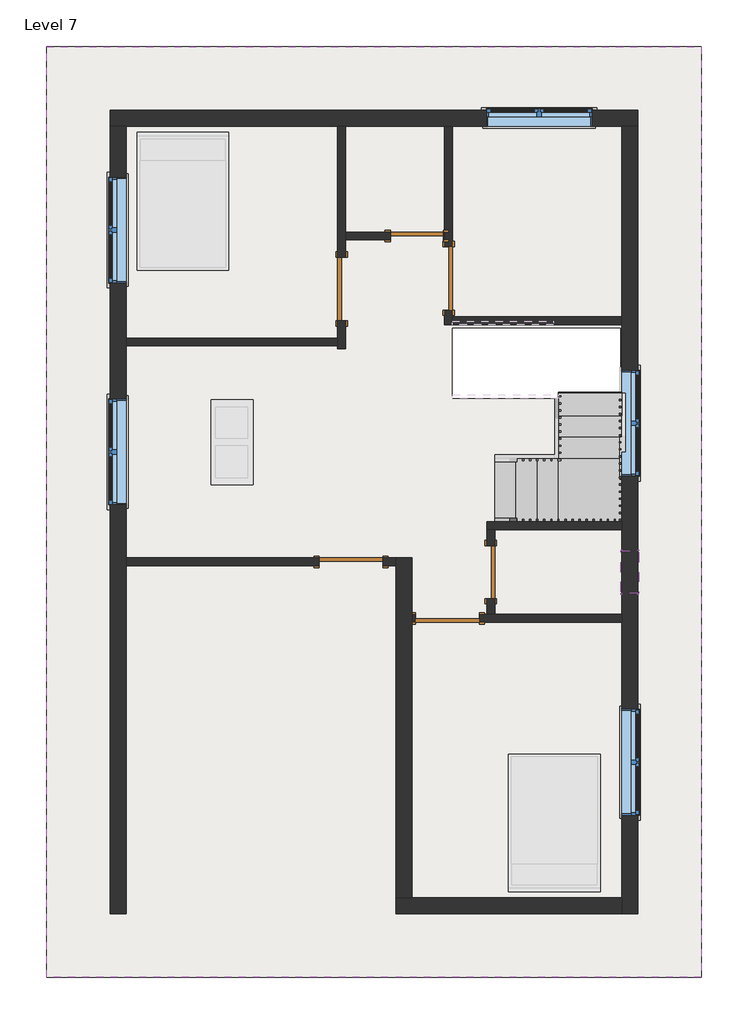
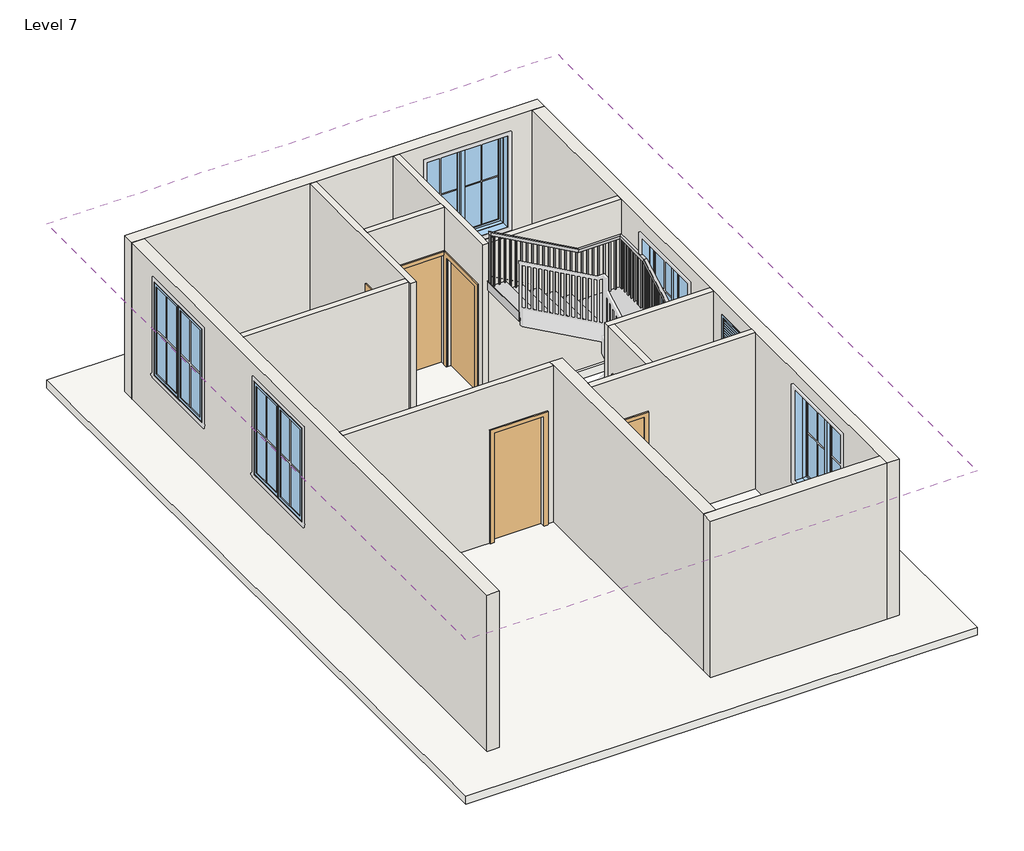
# One storey, part 1 of 2: 14 walls, 6 doors, 6 windows, 2 roofs, 1 railing, 1 slab, 1 stair flight.
# Revit data of these elements (continued)
# Elements 21, 22, 23, 24, 25 (IfcWall, "WALL 9\"")
#   Top Offset = 0' - 0"
#   Base Offset = 0' - 0"
#   Unconnected Height = 10' - 0"
#   wall height = 10' - 0"
#   Phase Created = New Construction
#   Base Constraint = Level 7
#   Materials on its faces: "Default Wall", "Copper"
# Element 26 (IfcWindow, "Window-Casement-Double : WIN 5'")
#   Mark = "31"
#   Window Inset = 0' - 0"
#   Interior Wall Closure = 0' - 2 1/4"
#   Frame Extension = 0' - 0 1/4"
#   Exterior Wall Closure = 0' - 1 1/4"
#   Interior Trim Visibility = yes
#   Exterior Trim Visibility = yes
#   Phase Created = New Construction
#   Materials on its faces: "Wood - Stained", "Glass", "Clad - White"
# Element 27 (IfcWindow, "Window-Casement-Double : WIN 5'")
#   Mark = "32"
#   Window Inset = 0' - 0"
#   Interior Wall Closure = 0' - 2 1/4"
#   Frame Extension = 0' - 0 1/4"
#   Exterior Wall Closure = 0' - 1 1/4"
#   Interior Trim Visibility = yes
#   Exterior Trim Visibility = yes
#   Phase Created = New Construction
#   Materials on its faces: "Wood - Stained", "Glass", "Clad - White"
# Element 28 (IfcWindow, "Window-Casement-Double : WIN 5'")
#   Mark = "33"
#   Window Inset = 0' - 0"
#   Interior Wall Closure = 0' - 2 1/4"
#   Frame Extension = 0' - 0 1/4"
#   Exterior Wall Closure = 0' - 1 1/4"
#   Interior Trim Visibility = yes
#   Exterior Trim Visibility = yes
#   Phase Created = New Construction
#   Materials on its faces: "Wood - Stained", "Glass", "Clad - White"
# Element 29 (IfcWindow, "Window-Casement-Double : WIN 5'")
#   Mark = "34"
#   Window Inset = 0' - 0"
#   Interior Wall Closure = 0' - 2 1/4"
#   Frame Extension = 0' - 0 1/4"
#   Exterior Wall Closure = 0' - 1 1/4"
#   Interior Trim Visibility = yes
#   Exterior Trim Visibility = yes
#   Phase Created = New Construction
#   Materials on its faces: "Wood - Stained", "Glass", "Clad - White"
# Element 30 (IfcWindow, "Window-Casement-Double : WIN 5'")
#   Mark = "35"
#   Window Inset = 0' - 0"
#   Interior Wall Closure = 0' - 2 1/4"
#   Frame Extension = 0' - 0 1/4"
#   Exterior Wall Closure = 0' - 1 1/4"
#   Interior Trim Visibility = yes
#   Exterior Trim Visibility = yes
#   Phase Created = New Construction
#   Materials on its faces: "Wood - Stained", "Glass", "Clad - White"
# Element 31 (IfcWindow, "Window-Louvers : 24\" x 24\"")
#   Mark = "36"
#   Blade Width = 1' - 10 1/2"
#   Phase Created = New Construction
#   Materials on its faces: "Birch"
# Materials
#   "Door - Panel": class "Wood", colour RGB 210 159 95, transparency 0, Cost = 0
#   "Door - Frame": colour RGB 118 70 51, transparency 0, Cost = 0
#   "Wood - Stained": class "Wood", colour RGB 224 178 126, transparency 0, Cost = 0
#   "Glass": class "Glass", colour RGB 0 128 192, transparency 0.75, Description = "Soda Lime Glass", Cost = 0
#   "Clad - White": class "Wood", colour RGB 242 242 238, transparency 0, Cost = 0
#   "Birch": class "Wood", colour RGB 224 178 126, transparency 0, Description = "Betula Alleghaniensis", Cost = 0
#   "Default Roof": colour RGB 88 101 114, transparency 0, Cost = 0
#   "Default Floor": colour RGB 128 128 128, transparency 0, Cost = 0
#   "Default Wall": colour RGB 128 128 128, transparency 0, Cost = 0
#   "Copper": class "Metal", colour RGB 0 0 0, transparency 0, Description = "Copper, matte finish", Cost = 0
